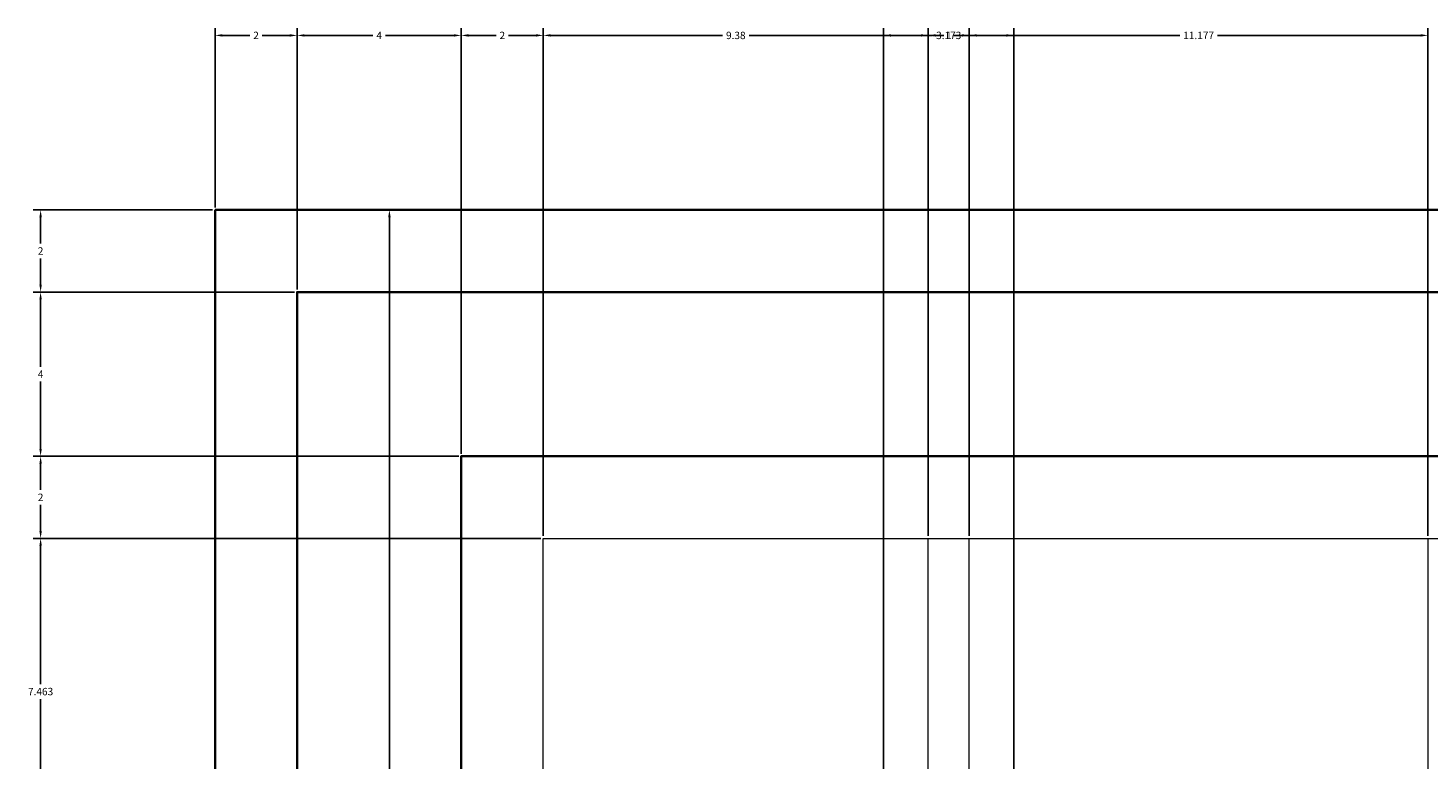
# Model space of a CAD drawing. Units: inches. Extents: x 3137 to 3299, y 1994 to 2089.
# Tile 6 of 14: x 3137 to 3171, y 2069 to 2087. Entities that reach past the tile are written whole.
import ezdxf

# ---------------------------------------------------------------- set-up
doc = ezdxf.new("R2010")
doc.units = ezdxf.units.IN
doc.header["$MEASUREMENT"] = 0
for name, color, linetype, lineweight in [('A-ANNO-DIMS', 2, 'Continuous', 18), ('A-ANNO-NPLT', 8, 'Continuous', 13), ('A-DOOR', 4, 'Continuous', 35), ('A-GLAZ', 3, 'Continuous', 18)]:
    doc.layers.add(name, color=color, linetype=linetype, lineweight=lineweight)
doc.styles.get("Standard").update_dxf_attribs({"font": 'arial.ttf'})
doc.dimstyles.get("Standard").update_dxf_attribs({"dimtxt": 0.18, "dimasz": 0.18, "dimexe": 0.18, "dimexo": 0.0625, "dimgap": 0.09, "dimtad": 0, "dimtih": 1, "dimtoh": 1, "dimdec": 4, "dimzin": 0, "dimdsep": 46, "dimtxsty": 'Standard', "dimcen": 0.09, "dimadec": 0, "dimazin": 0, "dimtfac": 1, "dimtdec": 4, "dimtofl": 0, "dimtmove": 0, "dimatfit": 3, "dimfxl": 1, "dimtolj": 1, "dimtzin": 0, "dimarcsym": 0})

# ---------------------------------------------------------------- blocks, each defined once
blk = doc.blocks.new('*D23')
at = {"layer": 'A-ANNO-DIMS', "color": 0, "lineweight": -2, "transparency": 16777216}
for p, q in [((3141.478, 2082.936), (3141.478, 2087.304)), ((3141.658, 2087.124), (3142.328, 2087.124)), ((3143.298, 2087.124), (3142.627, 2087.124)), ((3143.478, 2080.936), (3143.478, 2087.304))]:
    blk.add_line(p, q, dxfattribs=at)
at = {"layer": 'A-ANNO-DIMS', "color": 0, "transparency": 16777216}
for points in [[(3141.658, 2087.154), (3141.658, 2087.094), (3141.478, 2087.124)], [(3143.298, 2087.154), (3143.298, 2087.094), (3143.478, 2087.124)]]:
    blk.add_solid(points, dxfattribs=at)
at = {"layer": 'Defpoints', "color": 0, "transparency": 16777216}
for p in [(3143.478, 2087.124), (3141.478, 2082.874), (3143.478, 2080.874)]:
    blk.add_point(p, dxfattribs=at)
at = {"layer": 'A-ANNO-DIMS', "color": 0, "transparency": 16777216, "insert": (3142.478, 2087.124), "char_height": 0.18, "attachment_point": 5}
blk.add_mtext('\\A1;2', dxfattribs=at)
blk = doc.blocks.new('*D24')
at = {"layer": 'A-ANNO-DIMS', "color": 0, "lineweight": -2, "transparency": 16777216}
for p, q in [((3143.478, 2080.936), (3143.478, 2087.304)), ((3143.658, 2087.124), (3145.325, 2087.124)), ((3147.298, 2087.124), (3145.63, 2087.124)), ((3147.478, 2076.936), (3147.478, 2087.304))]:
    blk.add_line(p, q, dxfattribs=at)
at = {"layer": 'A-ANNO-DIMS', "color": 0, "transparency": 16777216}
for points in [[(3143.658, 2087.154), (3143.658, 2087.094), (3143.478, 2087.124)], [(3147.298, 2087.154), (3147.298, 2087.094), (3147.478, 2087.124)]]:
    blk.add_solid(points, dxfattribs=at)
at = {"layer": 'Defpoints', "color": 0, "transparency": 16777216}
for p in [(3147.478, 2087.124), (3143.478, 2080.874), (3147.478, 2076.874)]:
    blk.add_point(p, dxfattribs=at)
at = {"layer": 'A-ANNO-DIMS', "color": 0, "transparency": 16777216, "insert": (3145.478, 2087.124), "char_height": 0.18, "attachment_point": 5}
blk.add_mtext('\\A1;4', dxfattribs=at)
blk = doc.blocks.new('*D25')
at = {"layer": 'A-ANNO-DIMS', "color": 0, "lineweight": -2, "transparency": 16777216}
for p, q in [((3147.478, 2076.936), (3147.478, 2087.304)), ((3147.658, 2087.124), (3148.328, 2087.124)), ((3149.298, 2087.124), (3148.627, 2087.124)), ((3149.478, 2074.936), (3149.478, 2087.304))]:
    blk.add_line(p, q, dxfattribs=at)
at = {"layer": 'A-ANNO-DIMS', "color": 0, "transparency": 16777216}
for points in [[(3147.658, 2087.154), (3147.658, 2087.094), (3147.478, 2087.124)], [(3149.298, 2087.154), (3149.298, 2087.094), (3149.478, 2087.124)]]:
    blk.add_solid(points, dxfattribs=at)
at = {"layer": 'Defpoints', "color": 0, "transparency": 16777216}
for p in [(3149.478, 2087.124), (3147.478, 2076.874), (3149.478, 2074.874)]:
    blk.add_point(p, dxfattribs=at)
at = {"layer": 'A-ANNO-DIMS', "color": 0, "transparency": 16777216, "insert": (3148.478, 2087.124), "char_height": 0.18, "attachment_point": 5}
blk.add_mtext('\\A1;2', dxfattribs=at)
blk = doc.blocks.new('*D26')
at = {"layer": 'A-ANNO-DIMS', "color": 0, "lineweight": -2, "transparency": 16777216}
for p, q in [((3149.478, 2074.936), (3149.478, 2087.304)), ((3149.658, 2087.124), (3153.844, 2087.124)), ((3158.678, 2087.124), (3154.492, 2087.124)), ((3158.858, 2074.936), (3158.858, 2087.304))]:
    blk.add_line(p, q, dxfattribs=at)
at = {"layer": 'A-ANNO-DIMS', "color": 0, "transparency": 16777216}
for points in [[(3149.658, 2087.154), (3149.658, 2087.094), (3149.478, 2087.124)], [(3158.678, 2087.154), (3158.678, 2087.094), (3158.858, 2087.124)]]:
    blk.add_solid(points, dxfattribs=at)
at = {"layer": 'Defpoints', "color": 0, "transparency": 16777216}
for p in [(3158.858, 2087.124), (3149.478, 2074.874), (3158.858, 2074.874)]:
    blk.add_point(p, dxfattribs=at)
at = {"layer": 'A-ANNO-DIMS', "color": 0, "transparency": 16777216, "insert": (3154.168, 2087.124), "char_height": 0.18, "attachment_point": 5}
blk.add_mtext('\\A1;9.38', dxfattribs=at)
blk = doc.blocks.new('*D27')
at = {"layer": 'A-ANNO-DIMS', "color": 0, "lineweight": -2, "transparency": 16777216}
for p, q in [((3158.858, 2074.936), (3158.858, 2087.304)), ((3159.038, 2087.124), (3159.235, 2087.124)), ((3159.678, 2087.124), (3159.481, 2087.124)), ((3159.858, 2074.936), (3159.858, 2087.304))]:
    blk.add_line(p, q, dxfattribs=at)
at = {"layer": 'A-ANNO-DIMS', "color": 0, "transparency": 16777216}
for points in [[(3159.038, 2087.154), (3159.038, 2087.094), (3158.858, 2087.124)], [(3159.678, 2087.154), (3159.678, 2087.094), (3159.858, 2087.124)]]:
    blk.add_solid(points, dxfattribs=at)
at = {"layer": 'Defpoints', "color": 0, "transparency": 16777216}
for p in [(3159.858, 2087.124), (3158.858, 2074.874), (3159.858, 2074.874)]:
    blk.add_point(p, dxfattribs=at)
at = {"layer": 'A-ANNO-DIMS', "color": 0, "transparency": 16777216, "insert": (3159.358, 2087.124), "char_height": 0.18, "attachment_point": 5}
blk.add_mtext('\\A1;1', dxfattribs=at)
blk = doc.blocks.new('*D28')
at = {"layer": 'A-ANNO-DIMS', "color": 0, "lineweight": -2, "transparency": 16777216}
for p, q in [((3159.858, 2074.936), (3159.858, 2087.304)), ((3160.038, 2087.124), (3164.991, 2087.124)), ((3170.855, 2087.124), (3165.902, 2087.124)), ((3171.035, 2074.936), (3171.035, 2087.304))]:
    blk.add_line(p, q, dxfattribs=at)
at = {"layer": 'A-ANNO-DIMS', "color": 0, "transparency": 16777216}
for points in [[(3160.038, 2087.154), (3160.038, 2087.094), (3159.858, 2087.124)], [(3170.855, 2087.154), (3170.855, 2087.094), (3171.035, 2087.124)]]:
    blk.add_solid(points, dxfattribs=at)
at = {"layer": 'Defpoints', "color": 0, "transparency": 16777216}
for p in [(3171.035, 2087.124), (3159.858, 2074.874), (3171.035, 2074.874)]:
    blk.add_point(p, dxfattribs=at)
at = {"layer": 'A-ANNO-DIMS', "color": 0, "transparency": 16777216, "insert": (3165.446, 2087.124), "char_height": 0.18, "attachment_point": 5}
blk.add_mtext('\\A1;11.177', dxfattribs=at)
blk = doc.blocks.new('*D47')
at = {"layer": 'A-ANNO-DIMS', "color": 0, "lineweight": -2, "transparency": 16777216}
for p, q in [((3149.415, 2074.874), (3137.048, 2074.874)), ((3137.228, 2074.694), (3137.228, 2071.325)), ((3137.228, 2067.591), (3137.228, 2070.961)), ((3149.415, 2067.411), (3137.048, 2067.411))]:
    blk.add_line(p, q, dxfattribs=at)
at = {"layer": 'A-ANNO-DIMS', "color": 0, "transparency": 16777216}
for points in [[(3137.198, 2074.694), (3137.258, 2074.694), (3137.228, 2074.874)], [(3137.198, 2067.591), (3137.258, 2067.591), (3137.228, 2067.411)]]:
    blk.add_solid(points, dxfattribs=at)
at = {"layer": 'Defpoints', "color": 0, "transparency": 16777216}
for p in [(3137.228, 2074.874), (3149.478, 2074.874), (3149.478, 2067.411)]:
    blk.add_point(p, dxfattribs=at)
at = {"layer": 'A-ANNO-DIMS', "color": 0, "transparency": 16777216, "insert": (3137.228, 2071.143), "char_height": 0.18, "attachment_point": 5}
blk.add_mtext('\\A1;7.463', dxfattribs=at)
blk = doc.blocks.new('*D48')
at = {"layer": 'A-ANNO-DIMS', "color": 0, "lineweight": -2, "transparency": 16777216}
for p, q in [((3147.415, 2076.874), (3137.048, 2076.874)), ((3137.228, 2076.694), (3137.228, 2076.054)), ((3137.228, 2075.054), (3137.228, 2075.694)), ((3149.415, 2074.874), (3137.048, 2074.874))]:
    blk.add_line(p, q, dxfattribs=at)
at = {"layer": 'A-ANNO-DIMS', "color": 0, "transparency": 16777216}
for points in [[(3137.198, 2076.694), (3137.258, 2076.694), (3137.228, 2076.874)], [(3137.198, 2075.054), (3137.258, 2075.054), (3137.228, 2074.874)]]:
    blk.add_solid(points, dxfattribs=at)
at = {"layer": 'Defpoints', "color": 0, "transparency": 16777216}
for p in [(3137.228, 2076.874), (3147.478, 2076.874), (3149.478, 2074.874)]:
    blk.add_point(p, dxfattribs=at)
at = {"layer": 'A-ANNO-DIMS', "color": 0, "transparency": 16777216, "insert": (3137.228, 2075.874), "char_height": 0.18, "attachment_point": 5}
blk.add_mtext('\\A1;2', dxfattribs=at)
blk = doc.blocks.new('*D49')
at = {"layer": 'A-ANNO-DIMS', "color": 0, "lineweight": -2, "transparency": 16777216}
for p, q in [((3143.415181, 2080.873967), (3137.047681, 2080.873967)), ((3137.227681, 2080.693967), (3137.227681, 2079.053967)), ((3137.227681, 2077.053967), (3137.227681, 2078.693967)), ((3147.415181, 2076.873967), (3137.047681, 2076.873967))]:
    blk.add_line(p, q, dxfattribs=at)
at = {"layer": 'A-ANNO-DIMS', "color": 0, "transparency": 16777216}
for points in [[(3137.197681, 2080.693967), (3137.257681, 2080.693967), (3137.227681, 2080.873967)], [(3137.197681, 2077.053967), (3137.257681, 2077.053967), (3137.227681, 2076.873967)]]:
    blk.add_solid(points, dxfattribs=at)
at = {"layer": 'Defpoints', "color": 0, "transparency": 16777216}
for p in [(3137.227681, 2080.873967), (3143.477681, 2080.873967), (3147.477681, 2076.873967)]:
    blk.add_point(p, dxfattribs=at)
at = {"layer": 'A-ANNO-DIMS', "color": 0, "transparency": 16777216, "insert": (3137.227681, 2078.873967), "char_height": 0.18, "attachment_point": 5}
blk.add_mtext('\\A1;4', dxfattribs=at)
blk = doc.blocks.new('*D50')
at = {"layer": 'A-ANNO-DIMS', "color": 0, "lineweight": -2, "transparency": 16777216}
for p, q in [((3141.415, 2082.874), (3137.048, 2082.874)), ((3137.228, 2082.694), (3137.228, 2082.054)), ((3137.228, 2081.054), (3137.228, 2081.694)), ((3143.415, 2080.874), (3137.048, 2080.874))]:
    blk.add_line(p, q, dxfattribs=at)
at = {"layer": 'A-ANNO-DIMS', "color": 0, "transparency": 16777216}
for points in [[(3137.198, 2082.694), (3137.258, 2082.694), (3137.228, 2082.874)], [(3137.198, 2081.054), (3137.258, 2081.054), (3137.228, 2080.874)]]:
    blk.add_solid(points, dxfattribs=at)
at = {"layer": 'Defpoints', "color": 0, "transparency": 16777216}
for p in [(3137.228, 2082.874), (3141.478, 2082.874), (3143.478, 2080.874)]:
    blk.add_point(p, dxfattribs=at)
at = {"layer": 'A-ANNO-DIMS', "color": 0, "transparency": 16777216, "insert": (3137.228, 2081.874), "char_height": 0.18, "attachment_point": 5}
blk.add_mtext('\\A1;2', dxfattribs=at)
blk = doc.blocks.new('*D55')
at = {"layer": 'A-ANNO-DIMS', "color": 0, "lineweight": -2, "transparency": 16777216}
for p, q in [((3141.54, 2082.874), (3145.908, 2082.874)), ((3145.728, 2082.694), (3145.728, 2041.056)), ((3145.728, 1999.054), (3145.728, 2040.692)), ((3141.54, 1998.874), (3145.908, 1998.874))]:
    blk.add_line(p, q, dxfattribs=at)
at = {"layer": 'A-ANNO-DIMS', "color": 0, "transparency": 16777216}
for points in [[(3145.698, 2082.694), (3145.758, 2082.694), (3145.728, 2082.874)], [(3145.698, 1999.054), (3145.758, 1999.054), (3145.728, 1998.874)]]:
    blk.add_solid(points, dxfattribs=at)
at = {"layer": 'Defpoints', "color": 0, "transparency": 16777216}
for p in [(3141.478, 2082.874), (3141.478, 1998.874), (3145.728, 1998.874)]:
    blk.add_point(p, dxfattribs=at)
at = {"layer": 'A-ANNO-DIMS', "color": 0, "transparency": 16777216, "insert": (3145.728, 2040.874), "char_height": 0.18, "attachment_point": 5}
blk.add_mtext('\\A1;84', dxfattribs=at)
blk = doc.blocks.new('*D79')
at = {"layer": 'A-ANNO-DIMS', "color": 0, "lineweight": -2, "transparency": 16777216}
for p, q in [((3157.769, 2067.474), (3157.769, 2087.304)), ((3157.949, 2087.124), (3158.962, 2087.124)), ((3160.762, 2087.124), (3159.749, 2087.124)), ((3160.942, 2067.474), (3160.942, 2087.304))]:
    blk.add_line(p, q, dxfattribs=at)
at = {"layer": 'A-ANNO-DIMS', "color": 0, "transparency": 16777216}
for points in [[(3157.949, 2087.154), (3157.949, 2087.094), (3157.769, 2087.124)], [(3160.762, 2087.154), (3160.762, 2087.094), (3160.942, 2087.124)]]:
    blk.add_solid(points, dxfattribs=at)
at = {"layer": 'Defpoints', "color": 0, "transparency": 16777216}
for p in [(3160.942, 2087.124), (3157.769, 2067.411), (3160.942, 2067.411)]:
    blk.add_point(p, dxfattribs=at)
at = {"layer": 'A-ANNO-DIMS', "color": 0, "transparency": 16777216, "insert": (3159.356, 2087.124), "char_height": 0.18, "attachment_point": 5}
blk.add_mtext('\\A1;3.173', dxfattribs=at)

msp = doc.modelspace()

# ---------------------------------------------------------------- linework, layer by layer
at = {"layer": 'A-ANNO-NPLT'}
msp.add_point((3147.4777, 2076.874), dxfattribs=at)
at = {"layer": 'A-DOOR'}
for points in [[(3141.4777, 2082.874), (3189.4777, 2082.874), (3189.4777, 1998.874), (3141.4777, 1998.874)], [(3147.4777, 2056.9483), (3147.4777, 2076.874), (3183.4777, 2076.874), (3183.4777, 2056.9483)]]:
    msp.add_lwpolyline(points, close=True, dxfattribs=at)
msp.add_lwpolyline([(3187.4777, 2007.6773), (3187.4777, 2000.874), (3143.4777, 2000.874), (3143.4777, 2080.874), (3187.4777, 2080.874), (3187.4777, 2076.298)], dxfattribs=at)
at = {"layer": 'A-GLAZ'}
for p, q in [((3158.8577, 2068.3193), (3158.8577, 2074.874)), ((3159.8577, 2068.3193), (3159.8577, 2074.874)), ((3171.0351, 2068.3193), (3171.0351, 2074.874))]:
    msp.add_line(p, q, dxfattribs=at)
msp.add_lwpolyline([(3149.4777, 2058.9483), (3149.4777, 2074.874), (3181.4777, 2074.874), (3181.4777, 2058.9483)], close=True, dxfattribs=at)

# ---------------------------------------------------------------- dimensions: what is measured, and where the dimension line sits
at = {"layer": 'A-ANNO-DIMS'}
for base, p1, p2, override, picture, middle in [((3143.4777, 2087.124), (3141.4777, 2082.874), (3143.4777, 2080.874), {"dimdec": 0, "dimlfac": 1, "dimrnd": 0, "dimzin": 0, "dimdsep": 46, "dimlunit": 2}, '*D23', (3142.4777, 2087.124)), ((3147.4777, 2087.124), (3143.4777, 2080.874), (3147.4777, 2076.874), {"dimdec": 0, "dimlfac": 1, "dimrnd": 0, "dimzin": 0, "dimdsep": 46, "dimlunit": 2}, '*D24', (3145.4777, 2087.124)), ((3149.4777, 2087.124), (3147.4777, 2076.874), (3149.4777, 2074.874), {"dimdec": 0, "dimlfac": 1, "dimrnd": 0, "dimzin": 0, "dimdsep": 46, "dimlunit": 2}, '*D25', (3148.4777, 2087.124)), ((3158.8577, 2087.124), (3149.4777, 2074.874), (3158.8577, 2074.874), {"dimdec": 2, "dimlfac": 1, "dimrnd": 0, "dimzin": 0, "dimdsep": 46, "dimlunit": 2}, '*D26', (3154.1677, 2087.124)), ((3160.9422, 2087.124), (3157.7694, 2067.4111), (3160.9422, 2067.4111), {"dimdec": 3, "dimlfac": 1, "dimrnd": 0, "dimzin": 0, "dimdsep": 46, "dimlunit": 2}, '*D79', (3159.3558, 2087.124)), ((3159.8577, 2087.124), (3158.8577, 2074.874), (3159.8577, 2074.874), {"dimdec": 0, "dimlfac": 1, "dimrnd": 0, "dimzin": 0, "dimdsep": 46, "dimlunit": 2}, '*D27', (3159.3577, 2087.124)), ((3171.0351, 2087.124), (3159.8577, 2074.874), (3171.0351, 2074.874), {"dimdec": 3, "dimlfac": 1, "dimrnd": 0, "dimzin": 0, "dimdsep": 46, "dimlunit": 2}, '*D28', (3165.4464, 2087.124))]:
    dim = msp.add_linear_dim(base=base, p1=p1, p2=p2, dimstyle='Standard', override=override, dxfattribs=at)
    dim.commit()
    dim.dimension.update_dxf_attribs({"geometry": picture, "text_midpoint": middle})
for base, p1, p2, angle, override, picture, middle in [((3137.2277, 2082.874), (3143.4777, 2080.874), (3141.4777, 2082.874), 90, {"dimdec": 0, "dimlfac": 1, "dimrnd": 0, "dimzin": 0, "dimdsep": 46, "dimlunit": 2}, '*D50', (3137.2277, 2081.874)), ((3145.7277, 1998.874), (3141.4777, 2082.874), (3141.4777, 1998.874), 270, {"dimdec": 0, "dimlfac": 1, "dimrnd": 0, "dimzin": 0, "dimdsep": 46, "dimlunit": 2}, '*D55', (3145.7277, 2040.874)), ((3137.2277, 2080.874), (3147.4777, 2076.874), (3143.4777, 2080.874), 90, {"dimdec": 0, "dimlfac": 1, "dimrnd": 0, "dimzin": 0, "dimdsep": 46, "dimlunit": 2}, '*D49', (3137.2277, 2078.874)), ((3137.2277, 2076.874), (3149.4777, 2074.874), (3147.4777, 2076.874), 90, {"dimdec": 0, "dimlfac": 1, "dimrnd": 0, "dimzin": 0, "dimdsep": 46, "dimlunit": 2}, '*D48', (3137.2277, 2075.874)), ((3137.2277, 2074.874), (3149.4777, 2067.4111), (3149.4777, 2074.874), 90, {"dimdec": 3, "dimlfac": 1, "dimrnd": 0, "dimzin": 0, "dimdsep": 46, "dimlunit": 2}, '*D47', (3137.2277, 2071.1426))]:
    dim = msp.add_linear_dim(base=base, p1=p1, p2=p2, angle=angle, dimstyle='Standard', override=override, dxfattribs=at)
    dim.commit()
    dim.dimension.update_dxf_attribs({"geometry": picture, "text_midpoint": middle})

doc.saveas('drawing.dxf')
